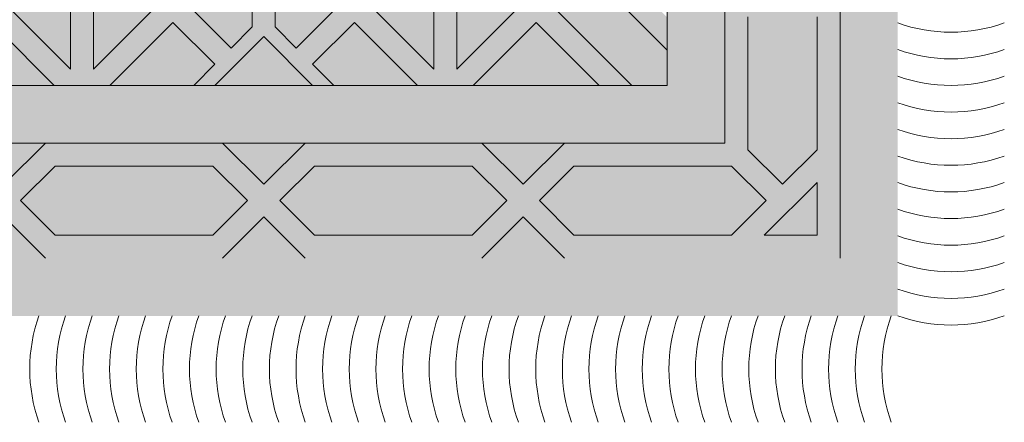
# Model space of a CAD drawing. Units: inches. Extents: x 844 to 2234, y 346 to 1084.
# Tile 53 of 93: x 1866.64 to 1877.53, y 688.07 to 692.53. Entities that reach past the tile are written whole.
import ezdxf

# ---------------------------------------------------------------- set-up
doc = ezdxf.new("R2010")
doc.units = ezdxf.units.IN
doc.header["$MEASUREMENT"] = 0
doc.layers.add('furniture', color=8, linetype='Continuous', lineweight=18)
doc.layers.add('RA-AP-01$0$INT', color=35, linetype='Continuous', lineweight=5)
doc.layers.add('RA-AP-01$0$FURN', color=3, linetype='Continuous')

# ---------------------------------------------------------------- blocks, each defined once
blk = doc.blocks.new('A$C18D01794')
at = {"layer": 'RA-AP-01$0$INT'}
h = blk.add_hatch(color=256, dxfattribs=at)
h.paths.add_polyline_path([(4.35521, -6.15671), (4.35521, -8.05671), (5.45521, -8.05671), (5.45521, -6.15671)])
h.paths.add_polyline_path([(4.40521, -8.00671), (4.40521, -6.20671), (5.40521, -6.20671), (5.40521, -8.00671)], flags=16)
h = blk.add_hatch(color=256, dxfattribs=at)
h.paths.add_polyline_path([(4.46935, -7.07085), (4.50521, -7.035), (4.50521, -7.10671)])
h.paths.add_polyline_path([(4.45521, -7.085), (4.47692, -7.10671), (4.43349, -7.10671)])
h.paths.add_polyline_path([(4.40521, -7.035), (4.44106, -7.07085), (4.40521, -7.10671)])
h.paths.add_polyline_path([(4.42521, -6.91146), (4.45521, -6.88146), (4.48521, -6.91146), (4.48521, -7.02671), (4.45521, -7.05671), (4.42521, -7.02671)])
h.paths.add_polyline_path([(4.50521, -6.83146), (4.50521, -6.90318), (4.46935, -6.86732)])
h.paths.add_polyline_path([(4.42521, -6.70793), (4.45521, -6.67793), (4.48521, -6.70793), (4.48521, -6.82318), (4.45521, -6.85318), (4.42521, -6.82318)])
h.paths.add_polyline_path([(4.42521, -6.50439), (4.45521, -6.47439), (4.48521, -6.50439), (4.48521, -6.61964), (4.45521, -6.64964), (4.42521, -6.61964)])
h.paths.add_polyline_path([(4.46935, -6.66378), (4.50521, -6.62793), (4.50521, -6.69964)])
h.paths.add_polyline_path([(4.40521, -6.62793), (4.44106, -6.66378), (4.40521, -6.69964)])
h.paths.add_polyline_path([(4.40521, -6.42439), (4.44106, -6.46025), (4.40521, -6.49611)])
h.paths.add_polyline_path([(4.46935, -6.46025), (4.50521, -6.42439), (4.50521, -6.49611)])
h.paths.add_polyline_path([(4.42521, -6.30085), (4.45521, -6.27085), (4.48521, -6.30085), (4.48521, -6.41611), (4.45521, -6.44611), (4.42521, -6.41611)])
h.paths.add_polyline_path([(4.42521, -6.22671), (4.47106, -6.22671), (4.42521, -6.27257)])
h.paths.add_polyline_path([(4.49935, -6.22671), (4.63606, -6.22671), (4.66606, -6.25671), (4.63606, -6.28671), (4.49935, -6.28671), (4.46935, -6.25671)])
h.paths.add_polyline_path([(4.68021, -6.27085), (4.71606, -6.30671), (4.64435, -6.30671)])
h.paths.add_polyline_path([(4.64435, -6.20671), (4.71606, -6.20671), (4.68021, -6.24257)])
h.paths.add_polyline_path([(4.72435, -6.22671), (4.86106, -6.22671), (4.89106, -6.25671), (4.86106, -6.28671), (4.72435, -6.28671), (4.69435, -6.25671)])
h.paths.add_polyline_path([(4.90521, -6.27085), (4.94106, -6.30671), (4.86935, -6.30671)])
h.paths.add_polyline_path([(4.86935, -6.20671), (4.94106, -6.20671), (4.90521, -6.24257)])
h.paths.add_polyline_path([(4.94935, -6.22671), (5.08606, -6.22671), (5.11606, -6.25671), (5.08606, -6.28671), (4.94935, -6.28671), (4.91935, -6.25671)])
h.paths.add_polyline_path([(5.13021, -6.27085), (5.16606, -6.30671), (5.09435, -6.30671)])
h.paths.add_polyline_path([(5.09435, -6.20671), (5.16606, -6.20671), (5.13021, -6.24257)])
h.paths.add_polyline_path([(5.17435, -6.22671), (5.31106, -6.22671), (5.34106, -6.25671), (5.31106, -6.28671), (5.17435, -6.28671), (5.14435, -6.25671)])
h.paths.add_polyline_path([(5.32521, -6.30085), (5.35521, -6.27085), (5.38521, -6.30085), (5.38521, -6.41611), (5.35521, -6.44611), (5.32521, -6.41611)])
h.paths.add_polyline_path([(5.33935, -6.22671), (5.38521, -6.22671), (5.38521, -6.27257)])
h.paths.add_polyline_path([(5.32521, -6.50439), (5.35521, -6.47439), (5.38521, -6.50439), (5.38521, -6.61964), (5.35521, -6.64964), (5.32521, -6.61964)])
h.paths.add_polyline_path([(5.30521, -6.42439), (5.34106, -6.46025), (5.30521, -6.49611)])
h.paths.add_polyline_path([(5.36935, -6.46025), (5.40521, -6.42439), (5.40521, -6.49611)])
h.paths.add_polyline_path([(5.40521, -6.62793), (5.40521, -6.69964), (5.36935, -6.66378)])
h.paths.add_polyline_path([(5.30521, -6.62793), (5.34106, -6.66378), (5.30521, -6.69964)])
h.paths.add_polyline_path([(5.32521, -6.70793), (5.35521, -6.67793), (5.38521, -6.70793), (5.38521, -6.82318), (5.35521, -6.85318), (5.32521, -6.82318)])
h.paths.add_polyline_path([(5.30521, -6.83146), (5.34106, -6.86732), (5.30521, -6.90318)])
h.paths.add_polyline_path([(5.32521, -6.91146), (5.35521, -6.88146), (5.38521, -6.91146), (5.38521, -7.02671), (5.35521, -7.05671), (5.32521, -7.02671)])
h.paths.add_polyline_path([(5.40458, -6.83209, 0.001218), (5.40521, -6.83231), (5.40521, -6.90318), (5.36935, -6.86732)])
h.paths.add_polyline_path([(5.36935, -7.07085), (5.40521, -7.035), (5.40521, -7.10671)])
h.paths.add_polyline_path([(5.35521, -7.085), (5.37692, -7.10671), (5.33349, -7.10671)])
h.paths.add_polyline_path([(5.30521, -7.035), (5.34106, -7.07085), (5.30521, -7.10671)])
h = blk.add_hatch(color=256, dxfattribs=at)
h.paths.add_polyline_path([(4.50521, -6.62793), (4.46935, -6.66378), (4.50521, -6.69964), (4.50521, -6.83146), (4.46935, -6.86732), (4.50521, -6.90318), (4.50521, -7.035), (4.46935, -7.07085), (4.50521, -7.10671), (4.47692, -7.10671), (4.45521, -7.085), (4.43349, -7.10671), (4.40521, -7.10671), (4.44106, -7.07085), (4.40521, -7.035), (4.40521, -6.90318), (4.44106, -6.86732), (4.40521, -6.83146), (4.40521, -6.69964), (4.44106, -6.66378), (4.40521, -6.62793), (4.40521, -6.49611), (4.44106, -6.46025), (4.40521, -6.42439), (4.40521, -6.20671), (4.64435, -6.20671), (4.68021, -6.24257), (4.71606, -6.20671), (4.86935, -6.20671), (4.90521, -6.24257), (4.94106, -6.20671), (5.09435, -6.20671), (5.13021, -6.24257), (5.16606, -6.20671), (5.40521, -6.20671), (5.40521, -6.42439), (5.36935, -6.46025), (5.40521, -6.49611), (5.40521, -6.62793), (5.36935, -6.66378), (5.40521, -6.69964), (5.40521, -6.83146), (5.36935, -6.86732), (5.40521, -6.90318), (5.40521, -7.035), (5.36935, -7.07085), (5.40521, -7.10671), (5.37692, -7.10671), (5.35521, -7.085), (5.33349, -7.10671), (5.30521, -7.10671), (5.34106, -7.07085), (5.30521, -7.035), (5.30521, -6.90318), (5.34106, -6.86732), (5.30521, -6.83146), (5.30521, -6.69964), (5.34106, -6.66378), (5.30521, -6.62793), (5.30521, -6.49611), (5.34106, -6.46025), (5.30521, -6.42439), (5.30521, -6.30671), (5.16606, -6.30671), (5.13021, -6.27085), (5.09435, -6.30671), (4.94106, -6.30671), (4.90521, -6.27085), (4.86935, -6.30671), (4.71606, -6.30671), (4.68021, -6.27085), (4.64435, -6.30671), (4.50521, -6.30671), (4.50521, -6.42439), (4.46935, -6.46025), (4.50521, -6.49611)])
h.paths.add_polyline_path([(4.48521, -6.50439), (4.45521, -6.47439), (4.42521, -6.50439), (4.42521, -6.61964), (4.45521, -6.64964), (4.48521, -6.61964)], flags=16)
h.paths.add_polyline_path([(4.45521, -6.44611), (4.48521, -6.41611), (4.48521, -6.30085), (4.45521, -6.27085), (4.42521, -6.30085), (4.42521, -6.41611)], flags=16)
h.paths.add_polyline_path([(4.45521, -6.67793), (4.42521, -6.70793), (4.42521, -6.82318), (4.45521, -6.85318), (4.48521, -6.82318), (4.48521, -6.70793)], flags=16)
h.paths.add_polyline_path([(4.49935, -6.28671), (4.63606, -6.28671), (4.66606, -6.25671), (4.63606, -6.22671), (4.49935, -6.22671), (4.46935, -6.25671)], flags=16)
h.paths.add_polyline_path([(4.42521, -6.27257), (4.47106, -6.22671), (4.42521, -6.22671)], flags=16)
h.paths.add_polyline_path([(4.45521, -6.88146), (4.42521, -6.91146), (4.42521, -7.02671), (4.45521, -7.05671), (4.48521, -7.02671), (4.48521, -6.91146)], flags=16)
h.paths.add_polyline_path([(4.72435, -6.28671), (4.86106, -6.28671), (4.89106, -6.25671), (4.86106, -6.22671), (4.72435, -6.22671), (4.69435, -6.25671)], flags=16)
h.paths.add_polyline_path([(4.91935, -6.25671), (4.94935, -6.28671), (5.08606, -6.28671), (5.11606, -6.25671), (5.08606, -6.22671), (4.94935, -6.22671)], flags=16)
h.paths.add_polyline_path([(5.14435, -6.25671), (5.17435, -6.28671), (5.31106, -6.28671), (5.34106, -6.25671), (5.31106, -6.22671), (5.17435, -6.22671)], flags=16)
h.paths.add_polyline_path([(5.32521, -6.61964), (5.35521, -6.64964), (5.38521, -6.61964), (5.38521, -6.50439), (5.35521, -6.47439), (5.32521, -6.50439)], flags=16)
h.paths.add_polyline_path([(5.32521, -6.41611), (5.35521, -6.44611), (5.38521, -6.41611), (5.38521, -6.30085), (5.35521, -6.27085), (5.32521, -6.30085)], flags=16)
h.paths.add_polyline_path([(5.32521, -6.70793), (5.32521, -6.82318), (5.35521, -6.85318), (5.38521, -6.82318), (5.38521, -6.70793), (5.35521, -6.67793)], flags=16)
h.paths.add_polyline_path([(5.32521, -6.91146), (5.32521, -7.02671), (5.35521, -7.05671), (5.38521, -7.02671), (5.38521, -6.91146), (5.35521, -6.88146)], flags=16)
h.paths.add_polyline_path([(5.33935, -6.22671), (5.38521, -6.27257), (5.38521, -6.22671)], flags=16)
blk.add_hatch(color=256, dxfattribs=at).paths.add_polyline_path([(4.50521, -6.30671), (5.30521, -6.30671), (5.30521, -7.10671), (5.25521, -7.10671), (5.25521, -6.35671), (4.55521, -6.35671), (4.55521, -7.10671), (4.50521, -7.10671)])
h = blk.add_hatch(color=256, dxfattribs=at)
h.paths.add_polyline_path([(4.58592, -6.35671), (4.55521, -6.35671), (4.55521, -6.38742), (4.8745, -6.70671), (4.90521, -6.676)])
h.paths.add_polyline_path([(5.25521, -6.38742), (5.25521, -6.35671), (5.2245, -6.35671), (4.90521, -6.676), (4.93592, -6.70671)])
h.paths.add_polyline_path([(4.93592, -6.70671), (4.90521, -6.73742), (5.25521, -7.08742), (5.25521, -7.026)])
h.paths.add_polyline_path([(4.55521, -7.026), (4.55521, -7.08742), (4.90521, -6.73742), (4.8745, -6.70671)])
h = blk.add_hatch(color=256, dxfattribs=at)
h.paths.add_polyline_path([(4.58592, -6.35671), (4.6142, -6.35671), (4.66885, -6.41136), (4.72349, -6.35671), (4.77177, -6.35671), (4.82642, -6.41136), (4.86278, -6.375), (4.8445, -6.35671), (4.86278, -6.35671), (4.90521, -6.39914), (4.94763, -6.35671), (4.96592, -6.35671), (4.94763, -6.375), (4.98399, -6.41136), (5.03864, -6.35671), (5.08692, -6.35671), (5.14157, -6.41136), (5.19621, -6.35671), (5.2245, -6.35671), (4.90521, -6.676)])
h.paths.add_polyline_path([(4.89521, -6.63772), (4.89521, -6.52843), (4.84056, -6.58307)], flags=16)
h.paths.add_polyline_path([(4.91521, -6.63772), (4.96985, -6.58307), (4.91521, -6.52843)], flags=16)
h.paths.add_polyline_path([(4.82642, -6.56893), (4.88106, -6.51429), (4.77177, -6.51429)], flags=16)
h.paths.add_polyline_path([(4.98399, -6.56893), (5.03864, -6.51429), (4.92935, -6.51429)], flags=16)
h.paths.add_polyline_path([(4.88106, -6.49429), (4.82642, -6.43964), (4.77177, -6.49429)], flags=16)
h.paths.add_polyline_path([(4.92935, -6.49429), (5.03864, -6.49429), (4.98399, -6.43964)], flags=16)
h.paths.add_polyline_path([(4.89521, -6.48014), (4.89521, -6.40742), (4.87692, -6.38914), (4.84056, -6.4255)], flags=16)
h.paths.add_polyline_path([(4.91521, -6.48014), (4.96985, -6.4255), (4.93349, -6.38914), (4.91521, -6.40742)], flags=16)
h.paths.add_polyline_path([(4.75763, -6.48014), (4.81228, -6.4255), (4.75763, -6.37085)], flags=16)
h.paths.add_polyline_path([(4.73763, -6.48014), (4.73763, -6.37085), (4.68299, -6.4255)], flags=16)
h.paths.add_polyline_path([(5.05278, -6.48014), (5.05278, -6.37085), (4.99814, -6.4255)], flags=16)
h.paths.add_polyline_path([(5.07278, -6.48014), (5.12742, -6.4255), (5.07278, -6.37085)], flags=16)
h.paths.add_polyline_path([(4.93592, -6.70671), (5.25521, -6.38742), (5.25521, -6.41571), (5.20056, -6.47035), (5.25521, -6.525), (5.25521, -6.57328), (5.20056, -6.62793), (5.23692, -6.66429), (5.25521, -6.646), (5.25521, -6.66429), (5.21278, -6.70671), (5.25521, -6.74914), (5.25521, -6.76742), (5.23692, -6.74914), (5.20056, -6.7855), (5.25521, -6.84014), (5.25521, -6.88843), (5.20056, -6.94307), (5.25521, -6.99772), (5.25521, -7.026)])
h.paths.add_polyline_path([(5.04299, -6.7855), (5.09763, -6.84014), (5.09763, -6.73085)], flags=16)
h.paths.add_polyline_path([(5.02885, -6.77136), (5.08349, -6.71671), (4.9742, -6.71671)], flags=16)
h.paths.add_polyline_path([(5.11763, -6.84014), (5.17228, -6.7855), (5.11763, -6.73085)], flags=16)
h.paths.add_polyline_path([(5.08349, -6.69671), (5.02885, -6.64207), (4.9742, -6.69671)], flags=16)
h.paths.add_polyline_path([(5.13177, -6.85429), (5.18642, -6.79964), (5.24106, -6.85429)], flags=17)
h.paths.add_polyline_path([(5.13177, -6.71671), (5.18642, -6.77136), (5.22278, -6.735), (5.2045, -6.71671)], flags=16)
h.paths.add_polyline_path([(5.09763, -6.68257), (5.09763, -6.57328), (5.04299, -6.62793)], flags=16)
h.paths.add_polyline_path([(5.13177, -6.87429), (5.24106, -6.87429), (5.18642, -6.92893)], flags=17)
h.paths.add_polyline_path([(5.13177, -6.69671), (5.2045, -6.69671), (5.22278, -6.67843), (5.18642, -6.64207)], flags=16)
h.paths.add_polyline_path([(5.11763, -6.68257), (5.17228, -6.62793), (5.11763, -6.57328)], flags=16)
h.paths.add_polyline_path([(5.18642, -6.61378), (5.24106, -6.55914), (5.13177, -6.55914)], flags=16)
h.paths.add_polyline_path([(5.13177, -6.53914), (5.24106, -6.53914), (5.18642, -6.48449)], flags=16)
h.paths.add_polyline_path([(5.25521, -7.08742), (5.25521, -7.10671), (4.55521, -7.10671), (4.55521, -7.08742), (4.90521, -6.73742)])
h.paths.add_polyline_path([(4.98399, -6.84449), (4.92935, -6.89914), (5.03864, -6.89914)], flags=16)
h.paths.add_polyline_path([(4.96985, -6.83035), (4.91521, -6.77571), (4.91521, -6.885)], flags=16)
h.paths.add_polyline_path([(4.92935, -6.91914), (4.98399, -6.97378), (5.03864, -6.91914)], flags=16)
h.paths.add_polyline_path([(5.05278, -6.93328), (4.99814, -6.98793), (5.05278, -7.04257)], flags=16)
h.paths.add_polyline_path([(5.07278, -6.93328), (5.07278, -7.04257), (5.12742, -6.98793)], flags=16)
h.paths.add_polyline_path([(4.89521, -6.77571), (4.84056, -6.83035), (4.89521, -6.885)], flags=16)
h.paths.add_polyline_path([(4.91521, -6.93328), (4.91521, -7.006), (4.93349, -7.02429), (4.96985, -6.98793)], flags=16)
h.paths.add_polyline_path([(4.88106, -6.89914), (4.82642, -6.84449), (4.77177, -6.89914)], flags=16)
h.paths.add_polyline_path([(4.89521, -6.93328), (4.84056, -6.98793), (4.87692, -7.02429), (4.89521, -7.006)], flags=16)
h.paths.add_polyline_path([(4.98399, -7.00207), (4.94763, -7.03843), (4.96592, -7.05671), (5.03864, -7.05671)], flags=16)
h.paths.add_polyline_path([(4.88106, -6.91914), (4.77177, -6.91914), (4.82642, -6.97378)], flags=16)
h.paths.add_polyline_path([(4.90521, -7.01429), (4.86278, -7.05671), (4.94763, -7.05671)], flags=16)
h.paths.add_polyline_path([(5.14157, -7.00207), (5.08692, -7.05671), (5.19621, -7.05671)], flags=16)
h.paths.add_polyline_path([(4.82642, -7.00207), (4.77177, -7.05671), (4.8445, -7.05671), (4.86278, -7.03843)], flags=16)
h.paths.add_polyline_path([(4.81228, -6.98793), (4.75763, -6.93328), (4.75763, -7.04257)], flags=16)
h.paths.add_polyline_path([(4.73763, -6.93328), (4.68299, -6.98793), (4.73763, -7.04257)], flags=16)
h.paths.add_polyline_path([(4.72349, -7.05671), (4.66885, -7.00207), (4.6142, -7.05671)], flags=16)
h.paths.add_polyline_path([(4.59763, -6.70671), (4.55521, -6.66429), (4.55521, -6.646), (4.57349, -6.66429), (4.60985, -6.62793), (4.55521, -6.57328), (4.55521, -6.525), (4.60985, -6.47035), (4.55521, -6.41571), (4.55521, -6.38742), (4.8745, -6.70671), (4.55521, -7.026), (4.55521, -6.99772), (4.60985, -6.94307), (4.55521, -6.88843), (4.55521, -6.84014), (4.60985, -6.7855), (4.57349, -6.74914), (4.55521, -6.76742), (4.55521, -6.74914)])
h.paths.add_polyline_path([(4.71278, -6.73085), (4.71278, -6.84014), (4.76742, -6.7855)], flags=16)
h.paths.add_polyline_path([(4.72692, -6.71671), (4.78157, -6.77136), (4.83621, -6.71671)], flags=16)
h.paths.add_polyline_path([(4.69278, -6.73085), (4.63814, -6.7855), (4.69278, -6.84014)], flags=16)
h.paths.add_polyline_path([(4.72692, -6.69671), (4.83621, -6.69671), (4.78157, -6.64207)], flags=16)
h.paths.add_polyline_path([(4.67864, -6.71671), (4.60592, -6.71671), (4.58763, -6.735), (4.62399, -6.77136)], flags=16)
h.paths.add_polyline_path([(4.71278, -6.68257), (4.76742, -6.62793), (4.71278, -6.57328)], flags=16)
h.paths.add_polyline_path([(4.67864, -6.69671), (4.62399, -6.64207), (4.58763, -6.67843), (4.60592, -6.69671)], flags=16)
h.paths.add_polyline_path([(4.69278, -6.68257), (4.69278, -6.57328), (4.63814, -6.62793)], flags=16)
h.paths.add_polyline_path([(4.62399, -6.79964), (4.67864, -6.85429), (4.56935, -6.85429)], flags=17)
h.paths.add_polyline_path([(4.62399, -6.61378), (4.67864, -6.55914), (4.56935, -6.55914)], flags=16)
h.paths.add_polyline_path([(4.67864, -6.87429), (4.62399, -6.92893), (4.56935, -6.87429)], flags=17)
h.paths.add_polyline_path([(4.67864, -6.53914), (4.62399, -6.48449), (4.56935, -6.53914)], flags=16)
h = blk.add_hatch(color=256, dxfattribs=at)
h.paths.add_polyline_path([(4.96985, -6.58307), (4.91521, -6.63772), (4.91521, -6.52843)])
h.paths.add_polyline_path([(4.89521, -6.63772), (4.84056, -6.58307), (4.89521, -6.52843)])
h.paths.add_polyline_path([(4.82642, -6.56893), (4.77177, -6.51429), (4.88106, -6.51429)])
h.paths.add_polyline_path([(4.88106, -6.49429), (4.77177, -6.49429), (4.82642, -6.43964)])
h.paths.add_polyline_path([(4.89521, -6.48014), (4.84056, -6.4255), (4.87692, -6.38914), (4.89521, -6.40742)])
h.paths.add_polyline_path([(4.86278, -6.375), (4.82642, -6.41136), (4.77177, -6.35671), (4.8445, -6.35671)])
h.paths.add_polyline_path([(4.81228, -6.4255), (4.75763, -6.48014), (4.75763, -6.37085)])
h.paths.add_polyline_path([(4.73763, -6.48014), (4.68299, -6.4255), (4.73763, -6.37085)])
h.paths.add_polyline_path([(4.66885, -6.41136), (4.6142, -6.35671), (4.72349, -6.35671)])
h.paths.add_polyline_path([(4.90521, -6.39914), (4.86278, -6.35671), (4.94763, -6.35671)])
h.paths.add_polyline_path([(4.91521, -6.48014), (4.91521, -6.40742), (4.93349, -6.38914), (4.96985, -6.4255)])
h.paths.add_polyline_path([(5.03864, -6.49429), (4.92935, -6.49429), (4.98399, -6.43964)])
h.paths.add_polyline_path([(4.98399, -6.56893), (4.92935, -6.51429), (5.03864, -6.51429)])
h.paths.add_polyline_path([(5.05278, -6.48014), (4.99814, -6.4255), (5.05278, -6.37085)])
h.paths.add_polyline_path([(4.98399, -6.41136), (4.94763, -6.375), (4.96592, -6.35671), (5.03864, -6.35671)])
h.paths.add_polyline_path([(5.12742, -6.4255), (5.07278, -6.48014), (5.07278, -6.37085)])
h.paths.add_polyline_path([(5.14157, -6.41136), (5.08692, -6.35671), (5.19621, -6.35671)])
for p, q in [((4.71606, -6.20671), (4.68021, -6.24257)), ((4.86935, -6.20671), (4.90521, -6.24257)), ((4.94106, -6.20671), (4.90521, -6.24257)), ((5.09435, -6.20671), (5.13021, -6.24257)), ((5.16606, -6.20671), (5.13021, -6.24257)), ((4.72435, -6.22671), (4.69435, -6.25671)), ((4.86106, -6.22671), (4.72435, -6.22671)), ((4.86106, -6.22671), (4.89106, -6.25671)), ((4.94935, -6.22671), (4.91935, -6.25671)), ((4.94935, -6.22671), (5.08606, -6.22671)), ((5.08606, -6.22671), (5.11606, -6.25671)), ((5.17435, -6.22671), (5.14435, -6.25671)), ((5.17435, -6.22671), (5.31106, -6.22671)), ((5.31106, -6.22671), (5.34106, -6.25671)), ((5.33935, -6.22671), (5.38521, -6.27257)), ((5.33935, -6.22671), (5.38521, -6.22671)), ((5.38521, -6.27257), (5.38521, -6.22671)), ((4.72435, -6.28671), (4.69435, -6.25671)), ((4.86106, -6.28671), (4.89106, -6.25671)), ((4.94935, -6.28671), (4.91935, -6.25671)), ((5.08606, -6.28671), (5.11606, -6.25671)), ((5.17435, -6.28671), (5.14435, -6.25671)), ((5.31106, -6.28671), (5.34106, -6.25671)), ((4.71606, -6.30671), (4.68021, -6.27085)), ((4.86935, -6.30671), (4.90521, -6.27085)), ((4.94106, -6.30671), (4.90521, -6.27085)), ((5.09435, -6.30671), (5.13021, -6.27085)), ((5.16606, -6.30671), (5.13021, -6.27085)), ((5.32521, -6.30085), (5.35521, -6.27085)), ((5.38521, -6.30085), (5.35521, -6.27085)), ((4.86106, -6.28671), (4.72435, -6.28671)), ((4.94935, -6.28671), (5.08606, -6.28671)), ((5.17435, -6.28671), (5.31106, -6.28671)), ((5.32521, -6.30085), (5.32521, -6.41611)), ((5.38521, -6.41611), (5.38521, -6.30085)), ((5.26721, -6.30671), (4.54321, -6.30671)), ((5.26721, -6.30671), (4.54321, -6.30671)), ((4.55521, -6.35671), (5.25521, -6.35671)), ((4.72349, -6.35671), (4.66885, -6.41136)), ((4.77177, -6.35671), (4.82642, -6.41136)), ((4.8445, -6.35671), (4.77177, -6.35671)), ((4.8445, -6.35671), (4.86278, -6.375)), ((4.94763, -6.35671), (4.86278, -6.35671)), ((4.90521, -6.39914), (4.86278, -6.35671)), ((4.90521, -6.39914), (4.94763, -6.35671)), ((4.90521, -6.676), (5.2245, -6.35671)), ((4.96592, -6.35671), (4.94763, -6.375)), ((4.94763, -6.375), (4.96592, -6.35671)), ((4.96592, -6.35671), (5.03864, -6.35671)), ((5.03864, -6.35671), (4.98399, -6.41136)), ((5.08692, -6.35671), (5.14157, -6.41136)), ((5.19621, -6.35671), (5.14157, -6.41136)), ((5.25521, -7.10671), (5.25521, -6.35671)), ((4.73763, -6.37085), (4.68299, -6.4255)), ((4.73763, -6.48014), (4.73763, -6.37085)), ((4.75763, -6.48014), (4.75763, -6.37085)), ((4.75763, -6.37085), (4.81228, -6.4255)), ((5.05278, -6.37085), (4.99814, -6.4255)), ((5.05278, -6.48014), (5.05278, -6.37085)), ((5.07278, -6.48014), (5.07278, -6.37085)), ((5.07278, -6.37085), (5.12742, -6.4255)), ((4.82642, -6.41136), (4.86278, -6.375)), ((4.98399, -6.41136), (4.94763, -6.375)), ((4.93592, -6.70671), (5.25521, -6.38742)), ((4.84056, -6.4255), (4.87692, -6.38914)), ((4.89521, -6.40742), (4.87692, -6.38914)), ((4.91521, -6.40742), (4.93349, -6.38914)), ((4.96985, -6.4255), (4.93349, -6.38914)), ((4.89521, -6.40742), (4.89521, -6.48014)), ((4.91521, -6.40742), (4.91521, -6.48014))]:
    blk.add_line(p, q, dxfattribs=at)
for points in [[(5.40521, -7.10671), (5.40521, -6.20671)], [(5.30521, -7.10671), (5.30521, -6.30671), (4.50521, -6.30671), (4.50521, -7.10671)]]:
    blk.add_lwpolyline(points, dxfattribs=at)
for centre, start, end in [((4.83866, -6.11051), 160.20384, 199.79616), ((4.86176, -6.11051), 160.20384, 199.79616), ((4.88486, -6.11051), 160.20384, 199.79616), ((4.90796, -6.11051), 160.20384, 199.79616), ((4.93106, -6.11051), 160.20384, 199.79616), ((4.95416, -6.11051), 160.20384, 199.79616), ((4.97726, -6.11051), 160.20384, 199.79616), ((5.00036, -6.11051), 160.20384, 199.79616), ((5.02346, -6.11051), 160.20384, 199.79616), ((5.04656, -6.11051), 160.20384, 199.79616), ((5.06966, -6.11051), 160.20384, 199.79616), ((5.09276, -6.11051), 160.20384, 199.79616), ((5.11586, -6.11051), 160.20384, 199.79616), ((5.13896, -6.11051), 160.20384, 199.79616), ((5.16206, -6.11051), 160.20384, 199.79616), ((5.18516, -6.11051), 160.20384, 199.79616), ((5.20826, -6.11051), 160.20384, 199.79616), ((5.23136, -6.11051), 160.20384, 199.79616), ((5.25446, -6.11051), 160.20384, 199.79616), ((5.27756, -6.11051), 160.20384, 199.79616), ((5.30066, -6.11051), 160.20384, 199.79616), ((5.32376, -6.11051), 160.20384, 199.79616), ((5.34686, -6.11051), 160.20384, 199.79616), ((5.36996, -6.11051), 160.20384, 199.79616), ((5.39306, -6.11051), 160.20384, 199.79616), ((5.41616, -6.11051), 160.20384, 199.79616), ((5.43926, -6.11051), 160.20384, 199.79616), ((5.46236, -6.11051), 160.20384, 199.79616), ((5.48546, -6.11051), 160.20384, 199.79616), ((5.50856, -6.11051), 160.20384, 199.79616), ((5.53166, -6.11051), 160.20384, 199.79616), ((5.55476, -6.11051), 160.20384, 199.79616), ((5.57786, -6.11051), 160.20384, 199.79616), ((5.50141, -6.28516), 70.20384, 109.79616), ((5.50141, -6.30826), 70.20384, 109.79616), ((5.50141, -6.33136), 70.20384, 109.79616), ((5.50141, -6.35446), 70.20384, 109.79616), ((5.50141, -6.37756), 70.20384, 109.79616), ((5.50141, -6.40066), 70.20384, 109.79616), ((5.50141, -6.42376), 70.20384, 109.79616), ((5.50141, -6.44686), 70.20384, 109.79616), ((5.50141, -6.46996), 70.20384, 109.79616), ((5.50141, -6.49306), 70.20384, 109.79616), ((5.50141, -6.51616), 70.20384, 109.79616), ((5.50141, -6.53926), 70.20384, 109.79616)]:
    blk.add_arc(centre, 0.13641, start, end, dxfattribs=at)
blk = doc.blocks.new('A$C5D2F253E')
at = {"layer": 'RA-AP-01$0$FURN', "xscale": -0.7999999999883585, "yscale": 0.7999999999883585, "zscale": 0.8, "rotation": 90}
blk.add_blockref('A$C18D01794', (-5.68776, 4.75792), dxfattribs=at)

msp = doc.modelspace()

# ---------------------------------------------------------------- block references
at = {"layer": 'furniture', "xscale": 15.94108302203742, "yscale": 15.94108302203742, "zscale": 15.94108302203742, "rotation": 90}
msp.add_blockref('A$C5D2F253E', (1882.631, 701.403), dxfattribs=at)

doc.saveas('drawing.dxf')
